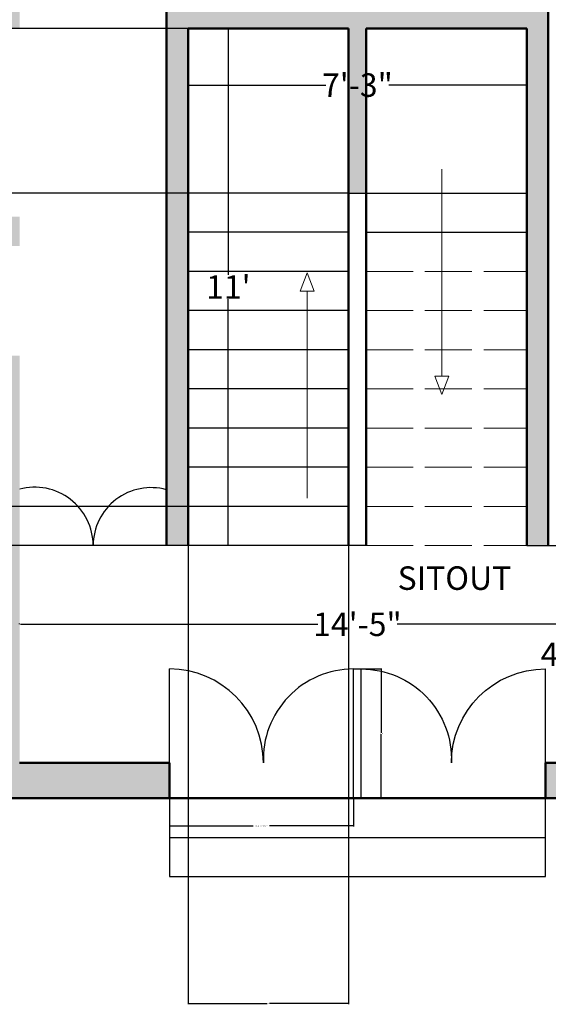
# Model space of a CAD drawing. Units: inches. Extents: x -28 to 544, y -640 to 52.
# Tile 2 of 11: x 162 to 297, y -640 to -389. Entities that reach past the tile are written whole.
import ezdxf

# ---------------------------------------------------------------- set-up
doc = ezdxf.new("R2010")
doc.units = ezdxf.units.IN
doc.header["$MEASUREMENT"] = 0
doc.linetypes.add('ACAD_ISO02W100', pattern=[15, 12, -3])
for name, color, linetype, lineweight in [('A-ANNO-DIMS', 2, 'Continuous', 18), ('A-ANNO-SYMB', 7, 'Continuous', 18), ('A-AREA-IDEN', 7, 'Continuous', 25), ('A-DOOR', 3, 'Continuous', 25), ('A-FLOR-STRS', 7, 'Continuous', 25), ('A-FLOR-STRS-HIDN', 8, 'ACAD_ISO02W100', 18), ('A-WALL', 7, 'Continuous', 50), ('A-WALL-PATT', 5, 'Continuous', 13)]:
    doc.layers.add(name, color=color, linetype=linetype, lineweight=lineweight)
doc.styles.get("Standard").update_dxf_attribs({"font": 'arial.ttf'})
doc.dimstyles.get("Standard").update_dxf_attribs({"dimtxt": 0.18, "dimasz": 0.18, "dimexe": 0.18, "dimexo": 0.0625, "dimgap": 0.09, "dimtad": 0, "dimtih": 1, "dimtoh": 1, "dimdec": 0, "dimzin": 0, "dimdsep": 46, "dimlunit": 3, "dimtxsty": 'Standard', "dimcen": 0.09, "dimadec": 0, "dimazin": 0, "dimtfac": 1, "dimtdec": 0, "dimtofl": 0, "dimtmove": 0, "dimatfit": 3, "dimfxl": 1, "dimtolj": 1, "dimtzin": 0, "dimarcsym": 0})

# ---------------------------------------------------------------- blocks, each defined once
blk = doc.blocks.new('*D33')
at = {"layer": 'A-ANNO-DIMS', "color": 0, "lineweight": -2, "transparency": 16777216}
for p, q in [((230.91, -391.24), (215.54, -391.24)), ((215.72, -391.42), (215.72, -454.14)), ((215.72, -523.06), (215.72, -460.34)), ((220.13, -523.24), (215.54, -523.24))]:
    blk.add_line(p, q, dxfattribs=at)
at = {"layer": 'A-ANNO-DIMS', "color": 0, "transparency": 16777216}
for points in [[(215.69, -391.42), (215.75, -391.42), (215.72, -391.24)], [(215.69, -523.06), (215.75, -523.06), (215.72, -523.24)]]:
    blk.add_solid(points, dxfattribs=at)
at = {"layer": 'Defpoints', "color": 0, "transparency": 16777216}
for p in [(215.72, -391.24), (230.97, -391.24), (220.19, -523.24)]:
    blk.add_point(p, dxfattribs=at)
at = {"layer": 'A-ANNO-DIMS', "color": 0, "transparency": 16777216, "insert": (215.72, -457.24), "char_height": 6, "attachment_point": 5}
blk.add_mtext("\\A1;11'", dxfattribs=at)
blk = doc.blocks.new('*D34')
at = {"layer": 'A-ANNO-DIMS', "color": 0, "lineweight": -2, "transparency": 16777216}
for p, q in [((205.44, -405.83), (205.44, -405.51)), ((205.62, -405.69), (240.65, -405.69)), ((291.76, -405.69), (256.73, -405.69)), ((291.94, -405.83), (291.94, -405.51))]:
    blk.add_line(p, q, dxfattribs=at)
at = {"layer": 'A-ANNO-DIMS', "color": 0, "transparency": 16777216}
for points in [[(205.62, -405.66), (205.62, -405.72), (205.44, -405.69)], [(291.76, -405.66), (291.76, -405.72), (291.94, -405.69)]]:
    blk.add_solid(points, dxfattribs=at)
at = {"layer": 'Defpoints', "color": 0, "transparency": 16777216}
for p in [(205.44, -405.9), (291.94, -405.69), (291.94, -405.9)]:
    blk.add_point(p, dxfattribs=at)
at = {"layer": 'A-ANNO-DIMS', "color": 0, "transparency": 16777216, "insert": (248.69, -405.69), "char_height": 6, "attachment_point": 5}
blk.add_mtext('\\A1;7\'-3"', dxfattribs=at)
blk = doc.blocks.new('*D41')
at = {"layer": 'A-ANNO-DIMS', "color": 0, "lineweight": -2, "transparency": 16777216}
for p, q in [((162.44, -543.27), (162.44, -543.15)), ((162.62, -543.33), (238.58, -543.33)), ((334.76, -543.33), (258.81, -543.33)), ((334.94, -543.27), (334.94, -543.15))]:
    blk.add_line(p, q, dxfattribs=at)
at = {"layer": 'A-ANNO-DIMS', "color": 0, "transparency": 16777216}
for points in [[(162.62, -543.3), (162.62, -543.36), (162.44, -543.33)], [(334.76, -543.3), (334.76, -543.36), (334.94, -543.33)]]:
    blk.add_solid(points, dxfattribs=at)
at = {"layer": 'Defpoints', "color": 0, "transparency": 16777216}
for p in [(162.44, -543.33), (334.94, -543.33), (334.94, -543.33)]:
    blk.add_point(p, dxfattribs=at)
at = {"layer": 'A-ANNO-DIMS', "color": 0, "transparency": 16777216, "insert": (248.69, -543.33), "char_height": 6, "attachment_point": 5}
blk.add_mtext('\\A1;14\'-5"', dxfattribs=at)
blk = doc.blocks.new('*D42')
at = {"layer": 'A-ANNO-DIMS', "color": 0, "lineweight": -2, "transparency": 16777216}
for p, q in [((297.51, -523.24), (304.73, -523.24)), ((304.55, -523.42), (304.55, -547.84)), ((304.55, -578.56), (304.55, -554.14)), ((301.15, -578.74), (304.73, -578.74))]:
    blk.add_line(p, q, dxfattribs=at)
at = {"layer": 'A-ANNO-DIMS', "color": 0, "transparency": 16777216}
for points in [[(304.52, -523.42), (304.58, -523.42), (304.55, -523.24)], [(304.52, -578.56), (304.58, -578.56), (304.55, -578.74)]]:
    blk.add_solid(points, dxfattribs=at)
at = {"layer": 'Defpoints', "color": 0, "transparency": 16777216}
for p in [(297.44, -523.24), (301.09, -578.74), (304.55, -578.74)]:
    blk.add_point(p, dxfattribs=at)
at = {"layer": 'A-ANNO-DIMS', "color": 0, "transparency": 16777216, "insert": (304.55, -550.99), "char_height": 6, "attachment_point": 5}
blk.add_mtext('\\A1;4\'-8"', dxfattribs=at)
blk = doc.blocks.new('STAIR-DIRECTION')
for p, q in [((1.81, 57.51), (1.81, 4.66)), ((1.81, 4.66), (0, 4.66)), ((0, 4.66), (1.81, 0)), ((1.81, 4.66), (3.63, 4.66)), ((3.63, 4.66), (1.81, 0))]:
    blk.add_line(p, q)
blk = doc.blocks.new('DOOR-ENTRY-PAIRED')
for p, q in [((0, 9), (0, 33)), ((47, 0), (47, 33))]:
    blk.add_line(p, q)
for centre, radius, start, end in [((0, 9), 24, 0, 90), ((47, 9.98), 23.02, 90, 182.4378)]:
    blk.add_arc(centre, radius, start, end)
blk = doc.blocks.new('*D79')
at = {"layer": 'A-ANNO-DIMS', "color": 0, "lineweight": -2, "transparency": 16777216}
for p, q in [((200.69, -587.8), (200.69, -594.97)), ((247.69, -587.8), (247.69, -594.97)), ((200.87, -594.79), (222.11, -594.79)), ((247.51, -594.79), (226.27, -594.79))]:
    blk.add_line(p, q, dxfattribs=at)
at = {"layer": 'A-ANNO-DIMS', "color": 0, "transparency": 16777216}
for points in [[(200.87, -594.76), (200.87, -594.82), (200.69, -594.79)], [(247.51, -594.76), (247.51, -594.82), (247.69, -594.79)]]:
    blk.add_solid(points, dxfattribs=at)
at = {"layer": 'Defpoints', "color": 0, "transparency": 16777216}
for p in [(200.69, -587.74), (247.69, -587.74), (247.69, -594.79)]:
    blk.add_point(p, dxfattribs=at)
at = {"layer": 'A-ANNO-DIMS', "color": 0, "transparency": 16777216, "insert": (224.19, -594.79), "char_height": 0.18, "attachment_point": 5}
blk.add_mtext('\\A1;PAIRED ENTRY DOOR 3\'-11" TYP.', dxfattribs=at)
blk = doc.blocks.new('*D80')
at = {"layer": 'A-ANNO-DIMS', "color": 0, "lineweight": -2, "transparency": 16777216}
for p, q in [((247.76, -554.74), (254.92, -554.74)), ((254.74, -554.92), (254.74, -571.06)), ((254.74, -587.56), (254.74, -571.42)), ((247.76, -587.74), (254.92, -587.74))]:
    blk.add_line(p, q, dxfattribs=at)
at = {"layer": 'A-ANNO-DIMS', "color": 0, "transparency": 16777216}
for points in [[(254.71, -554.92), (254.77, -554.92), (254.74, -554.74)], [(254.71, -587.56), (254.77, -587.56), (254.74, -587.74)]]:
    blk.add_solid(points, dxfattribs=at)
at = {"layer": 'Defpoints', "color": 0, "transparency": 16777216}
for p in [(247.69, -554.74), (254.74, -554.74), (247.69, -587.74)]:
    blk.add_point(p, dxfattribs=at)
at = {"layer": 'A-ANNO-DIMS', "color": 0, "transparency": 16777216, "insert": (254.74, -571.24), "char_height": 0.18, "attachment_point": 5}
blk.add_mtext('\\A1;2\'-9" TYP.', dxfattribs=at)
blk = doc.blocks.new('*D81')
at = {"layer": 'A-ANNO-DIMS', "color": 0, "lineweight": -2, "transparency": 16777216}
for p, q in [((205.44, -523.3), (205.44, -640.35)), ((246.44, -523.3), (246.44, -640.35)), ((205.62, -640.17), (225.62, -640.17)), ((246.26, -640.17), (226.27, -640.17))]:
    blk.add_line(p, q, dxfattribs=at)
at = {"layer": 'A-ANNO-DIMS', "color": 0, "transparency": 16777216}
for points in [[(205.62, -640.14), (205.62, -640.2), (205.44, -640.17)], [(246.26, -640.14), (246.26, -640.2), (246.44, -640.17)]]:
    blk.add_solid(points, dxfattribs=at)
at = {"layer": 'Defpoints', "color": 0, "transparency": 16777216}
for p in [(205.44, -523.24), (246.44, -523.24), (246.44, -640.17)]:
    blk.add_point(p, dxfattribs=at)
at = {"layer": 'A-ANNO-DIMS', "color": 0, "transparency": 16777216, "insert": (225.94, -640.17), "char_height": 0.18, "attachment_point": 5}
blk.add_mtext('\\A1;3\'-5"', dxfattribs=at)
blk = doc.blocks.new('*D82')
at = {"layer": 'A-ANNO-DIMS', "color": 0, "lineweight": -2, "transparency": 16777216}
for p, q in [((205.38, -513.24), (-27.66, -513.24)), ((-27.48, -513.42), (-27.48, -518.06)), ((-27.48, -523.06), (-27.48, -518.42)), ((205.38, -523.24), (-27.66, -523.24))]:
    blk.add_line(p, q, dxfattribs=at)
at = {"layer": 'A-ANNO-DIMS', "color": 0, "transparency": 16777216}
for points in [[(-27.51, -513.42), (-27.45, -513.42), (-27.48, -513.24)], [(-27.51, -523.06), (-27.45, -523.06), (-27.48, -523.24)]]:
    blk.add_solid(points, dxfattribs=at)
at = {"layer": 'Defpoints', "color": 0, "transparency": 16777216}
for p in [(-27.48, -513.24), (205.44, -513.24), (205.44, -523.24)]:
    blk.add_point(p, dxfattribs=at)
at = {"layer": 'A-ANNO-DIMS', "color": 0, "transparency": 16777216, "insert": (-27.48, -518.24), "char_height": 0.18, "attachment_point": 5}
blk.add_mtext('\\A1;0\'-10"', dxfattribs=at)
blk = doc.blocks.new('*D83')
at = {"layer": 'A-ANNO-DIMS', "color": 0, "lineweight": -2, "transparency": 16777216}
for p, q in [((205.38, -391.24), (-27.66, -391.24)), ((-27.48, -391.42), (-27.48, -412.06)), ((-27.48, -433.06), (-27.48, -412.42)), ((205.38, -433.24), (-27.66, -433.24))]:
    blk.add_line(p, q, dxfattribs=at)
at = {"layer": 'A-ANNO-DIMS', "color": 0, "transparency": 16777216}
for points in [[(-27.51, -391.42), (-27.45, -391.42), (-27.48, -391.24)], [(-27.51, -433.06), (-27.45, -433.06), (-27.48, -433.24)]]:
    blk.add_solid(points, dxfattribs=at)
at = {"layer": 'Defpoints', "color": 0, "transparency": 16777216}
for p in [(205.44, -391.24), (-27.48, -433.24), (205.44, -433.24)]:
    blk.add_point(p, dxfattribs=at)
at = {"layer": 'A-ANNO-DIMS', "color": 0, "transparency": 16777216, "insert": (-27.48, -412.24), "char_height": 0.18, "attachment_point": 5}
blk.add_mtext('\\A1;3\'-6"', dxfattribs=at)

msp = doc.modelspace()

# ---------------------------------------------------------------- hatches: boundary and pattern name
at = {"layer": 'A-WALL-PATT'}
h = msp.add_hatch(color=256, dxfattribs=at)
h.dxf.hatch_style = 1
h.paths.add_polyline_path([(25.94, -235.24), (16.94, -235.24), (16.94, -290.74), (25.94, -290.74), (25.94, -254.74), (127.94, -254.74), (127.94, -252.49), (127.94, -250.24), (118.94, -250.24), (118.94, -247.24), (109.94, -247.24), (109.94, -250.24), (25.94, -250.24)])
h.paths.add_polyline_path([(114.44, -191.74), (114.44, -137.74), (126.94, -137.74), (126.94, -135.49), (126.94, -133.24), (109.94, -133.24), (109.94, -137.74), (109.94, -191.74), (25.94, -191.74), (25.94, -176.74), (16.94, -176.74), (16.94, -211.24), (25.94, -211.24), (25.94, -196.24), (109.94, -196.24), (109.94, -219.24), (114.44, -219.24), (114.44, -196.24)])
h.paths.add_polyline_path([(25.94, -350.74), (16.94, -350.74), (16.94, -403.24), (25.94, -403.24), (25.94, -391.24), (121.94, -391.24), (121.94, -403.24), (126.44, -403.24), (126.44, -391.24), (162.44, -391.24), (162.44, -250.24), (155.94, -250.24), (155.94, -254.74), (157.94, -254.74), (157.94, -386.74), (25.94, -386.74)])
h.paths.add_polyline_path([(25.94, -443.74), (157.94, -443.74), (157.94, -446.74), (162.44, -446.74), (162.44, -439.24), (126.44, -439.24), (126.44, -427.74), (121.94, -427.74), (121.94, -439.24), (25.94, -439.24), (25.94, -427.24), (16.94, -427.24), (16.94, -481.24), (25.94, -481.24)])
h.paths.add_polyline_path([(25.94, -541.24), (16.94, -541.24), (16.94, -587.74), (61.94, -587.74), (61.94, -578.74), (25.94, -578.74)])
h.paths.add_polyline_path([(162.44, -578.74), (162.44, -474.74), (160.19, -474.74), (157.94, -474.74), (157.94, -578.74), (121.94, -578.74), (121.94, -587.74), (162.44, -587.74)])
h.paths.add_polyline_path([(200.69, -578.74), (162.44, -578.74), (162.44, -587.74), (200.69, -587.74)])
h.paths.add_polyline_path([(25.94, -97.24), (16.94, -97.24), (16.94, -152.74), (25.94, -152.74), (25.94, -137.74), (81.94, -137.74), (81.94, -135.49), (81.94, -133.24), (25.94, -133.24)])
h.paths.add_polyline_path([(210.44, -133.24), (162.44, -133.24), (162.44, -1.24), (186.44, -1.24), (186.44, 7.76), (121.94, 7.76), (121.94, -1.24), (157.94, -1.24), (157.94, -133.24), (154.94, -133.24), (154.94, -137.74), (210.44, -137.74)])
h.paths.add_polyline_path([(61.94, 7.76), (16.94, 7.76), (16.94, -37.24), (25.94, -37.24), (25.94, -1.24), (61.94, -1.24)])
h = msp.add_hatch(color=256, dxfattribs=at)
h.dxf.hatch_style = 1
h.paths.add_polyline_path([(375.44, 7.76), (310.94, 7.76), (310.94, -1.24), (334.94, -1.24), (334.94, -133.24), (286.94, -133.24), (286.94, -137.74), (342.44, -137.74), (342.44, -133.24), (339.44, -133.24), (339.44, -1.24), (375.44, -1.24)])
h.paths.add_polyline_path([(480.44, 7.76), (435.44, 7.76), (435.44, -1.24), (471.44, -1.24), (471.44, -37.24), (480.44, -37.24)])
h.paths.add_polyline_path([(480.44, -97.24), (471.44, -97.24), (471.44, -133.24), (417.44, -133.24), (417.44, -135.49), (417.44, -137.74), (471.44, -137.74), (471.44, -152.74), (480.44, -152.74)])
h.paths.add_polyline_path([(480.44, -176.74), (471.44, -176.74), (471.44, -191.74), (387.44, -191.74), (387.44, -137.74), (389.44, -137.74), (389.44, -133.24), (370.44, -133.24), (370.44, -135.49), (370.44, -137.74), (382.94, -137.74), (382.94, -191.74), (382.94, -196.24), (382.94, -220.24), (385.19, -220.24), (387.44, -220.24), (387.44, -196.24), (471.44, -196.24), (471.44, -211.24), (480.44, -211.24)])
h.paths.add_polyline_path([(480.44, -235.24), (471.44, -235.24), (471.44, -250.24), (387.44, -250.24), (387.44, -248.24), (382.94, -248.24), (382.94, -250.24), (369.44, -250.24), (369.44, -252.49), (369.44, -254.74), (471.44, -254.74), (471.44, -290.74), (480.44, -290.74)])
h.paths.add_polyline_path([(480.44, -350.74), (471.44, -350.74), (471.44, -386.74), (339.44, -386.74), (339.44, -254.74), (341.44, -254.74), (341.44, -250.24), (334.94, -250.24), (334.94, -391.24), (471.44, -391.24), (471.44, -403.24), (480.44, -403.24)])
h.paths.add_polyline_path([(480.44, -427.24), (471.44, -427.24), (471.44, -439.24), (334.94, -439.24), (334.94, -446.74), (339.44, -446.74), (339.44, -443.74), (471.44, -443.74), (471.44, -481.24), (480.44, -481.24)])
h.paths.add_polyline_path([(480.44, -541.24), (471.44, -541.24), (471.44, -578.74), (435.44, -578.74), (435.44, -587.74), (480.44, -587.74)])
h.paths.add_polyline_path([(375.44, -578.74), (339.44, -578.74), (339.44, -474.74), (337.19, -474.74), (334.94, -474.74), (334.94, -578.74), (296.69, -578.74), (296.69, -587.74), (375.44, -587.74)])
h = msp.add_hatch(color=256, dxfattribs=at)
h.dxf.hatch_style = 1
h.paths.add_polyline_path([(246.44, -386.74), (199.94, -386.74), (199.94, -391.24), (199.94, -523.24), (205.44, -523.24), (205.44, -391.24), (246.44, -391.24), (246.44, -433.24), (250.94, -433.24), (250.94, -391.24), (291.94, -391.24), (291.94, -523.24), (297.44, -523.24), (297.44, -386.74), (250.94, -386.74), (250.94, -250.24), (246.44, -250.24)])
h.paths.add_polyline_path([(244.06, -411.97), (253.32, -411.97), (253.32, -399.6), (244.06, -399.6)], flags=25)

# ---------------------------------------------------------------- linework, layer by layer
at = {"layer": 'A-DOOR'}
msp.add_line((224.69, -578.74), (224.69, -578.74), dxfattribs=at)
for centre, radius, start, end in [((166.3, -523.24), 14.9, 360, 104.9905), ((195.99, -523.24), 14.79, 74.4943, 180)]:
    msp.add_arc(centre, radius, start, end, dxfattribs=at)
at = {"layer": 'A-FLOR-STRS'}
for p, q in [((246.44, -433.24), (205.44, -433.24)), ((246.44, -433.24), (291.94, -433.24)), ((246.44, -443.24), (205.44, -443.24)), ((250.94, -443.24), (291.94, -443.24)), ((246.44, -453.24), (205.44, -453.24)), ((246.44, -463.24), (205.44, -463.24)), ((246.44, -473.24), (205.44, -473.24)), ((246.44, -483.24), (205.44, -483.24)), ((246.44, -493.24), (205.44, -493.24)), ((246.44, -503.24), (205.44, -503.24)), ((246.44, -513.24), (205.44, -513.24)), ((250.94, -523.24), (199.94, -523.24)), ((291.94, -523.24), (297.44, -523.24)), ((200.69, -587.74), (200.69, -597.74)), ((296.69, -607.74), (296.69, -587.74)), ((200.69, -597.74), (200.69, -607.74)), ((200.69, -597.74), (296.69, -597.74)), ((200.69, -607.74), (296.69, -607.74))]:
    msp.add_line(p, q, dxfattribs=at)
at = {"layer": 'A-FLOR-STRS-HIDN'}
for p, q in [((250.94, -453.24), (291.94, -453.24)), ((250.94, -463.24), (291.94, -463.24)), ((250.94, -473.24), (291.94, -473.24)), ((250.94, -483.24), (291.94, -483.24)), ((250.94, -493.24), (291.94, -493.24)), ((250.94, -503.24), (291.94, -503.24)), ((250.94, -513.24), (291.94, -513.24)), ((250.94, -523.24), (291.94, -523.24))]:
    msp.add_line(p, q, dxfattribs=at)
at = {"layer": 'A-WALL'}
for p, q in [((199.94, -391.24), (199.94, -386.74)), ((297.44, -523.24), (297.44, -386.74)), ((199.94, -523.24), (199.94, -391.24)), ((246.44, -391.24), (205.44, -391.24)), ((205.44, -391.24), (205.44, -523.24)), ((246.44, -391.24), (246.44, -523.24)), ((250.94, -391.24), (250.94, -523.24)), ((250.94, -391.24), (291.94, -391.24)), ((291.94, -391.24), (291.94, -523.24)), ((162.44, -578.74), (200.69, -578.74)), ((200.69, -578.74), (200.69, -587.74)), ((296.69, -578.74), (334.94, -578.74)), ((296.69, -578.74), (296.69, -587.74)), ((16.94, -587.74), (480.44, -587.74))]:
    msp.add_line(p, q, dxfattribs=at)

# ---------------------------------------------------------------- block references
at = {"layer": 'A-ANNO-SYMB'}
msp.add_blockref('STAIR-DIRECTION', (268.43, -484.64), dxfattribs=at)
at = {"layer": 'A-ANNO-SYMB', "rotation": 180}
msp.add_blockref('STAIR-DIRECTION', (237.69, -453.64), dxfattribs=at)
at = {"layer": 'A-DOOR'}
msp.add_blockref('DOOR-ENTRY-PAIRED', (200.69, -587.74), dxfattribs=at)
at = {"layer": 'A-DOOR', "extrusion": (0, 0, -1), "zscale": -1}
msp.add_blockref('DOOR-ENTRY-PAIRED', (-296.69, -587.74), dxfattribs=at)

# ---------------------------------------------------------------- texts
at = {"layer": 'A-AREA-IDEN', "insert": (258.95, -528.55), "char_height": 6, "attachment_point": 1}
msp.add_mtext('SITOUT', dxfattribs=at)

# ---------------------------------------------------------------- dimensions: what is measured, and where the dimension line sits
at = {"layer": 'A-ANNO-DIMS'}
for base, p1, p2, override, picture, middle in [((-27.48, -433.24), (205.44, -391.24), (205.44, -433.24), {"dimdec": 1, "dimlfac": 1, "dimrnd": 0, "dimzin": 1, "dimdsep": 46, "dimlunit": 4, "dimfrac": 2}, '*D83', (-27.48, -412.24)), ((215.72, -391.24), (220.19, -523.24), (230.97, -391.24), {"dimtxt": 6, "dimclrd": 0, "dimclre": 0, "dimclrt": 0}, '*D33', (215.72, -457.24)), ((-27.48, -513.24), (205.44, -523.24), (205.44, -513.24), {"dimdec": 1, "dimlfac": 1, "dimrnd": 0, "dimzin": 1, "dimdsep": 46, "dimlunit": 4, "dimfrac": 2}, '*D82', (-27.48, -518.24)), ((304.55174986, -578.74117838), (297.44473605, -523.24117838), (301.09042073, -578.74117838), {"dimtxt": 6, "dimclrd": 0, "dimclre": 0, "dimclrt": 0}, '*D42', (304.55174986, -550.99117838))]:
    dim = msp.add_linear_dim(base=base, p1=p1, p2=p2, angle=90, dimstyle='Standard', override=override, dxfattribs=at)
    dim.commit()
    dim.dimension.update_dxf_attribs({"geometry": picture, "text_midpoint": middle})
for base, p1, p2, override, picture, middle in [((291.94473605, -405.6923478), (205.44473605, -405.89650751), (291.94473605, -405.89650751), {"dimtxt": 6, "dimclrd": 0, "dimclre": 0, "dimclrt": 0}, '*D34', (248.69473605, -405.6923478)), ((246.44, -640.17), (205.44, -523.24), (246.44, -523.24), {"dimdec": 1, "dimlfac": 1, "dimrnd": 0, "dimzin": 1, "dimdsep": 46, "dimlunit": 4, "dimfrac": 2}, '*D81', (225.94, -640.17)), ((334.94473605, -543.33075676), (162.44473605, -543.33075676), (334.94473605, -543.33075676), {"dimtxt": 6, "dimclrd": 0, "dimclre": 0, "dimclrt": 0}, '*D41', (248.69473605, -543.33075676))]:
    dim = msp.add_linear_dim(base=base, p1=p1, p2=p2, dimstyle='Standard', override=override, dxfattribs=at)
    dim.commit()
    dim.dimension.update_dxf_attribs({"geometry": picture, "text_midpoint": middle})
dim = msp.add_linear_dim(base=(254.74, -554.74), p1=(247.69, -587.74), p2=(247.69, -554.74), angle=90, text='<> TYP.', dimstyle='Standard', override={"dimdec": 1, "dimlfac": 1, "dimrnd": 0, "dimzin": 1, "dimdsep": 46, "dimlunit": 4, "dimfrac": 2}, dxfattribs=at)
dim.commit()
dim.dimension.update_dxf_attribs({"geometry": '*D80', "text_midpoint": (254.74, -571.24)})
dim = msp.add_linear_dim(base=(247.69, -594.79), p1=(200.69, -587.74), p2=(247.69, -587.74), text='PAIRED ENTRY DOOR <> TYP.', dimstyle='Standard', override={"dimdec": 1, "dimlfac": 1, "dimrnd": 0, "dimzin": 1, "dimdsep": 46, "dimlunit": 4, "dimfrac": 2}, dxfattribs=at)
dim.commit()
dim.dimension.update_dxf_attribs({"geometry": '*D79', "text_midpoint": (224.19, -594.79)})

doc.saveas('drawing.dxf')
